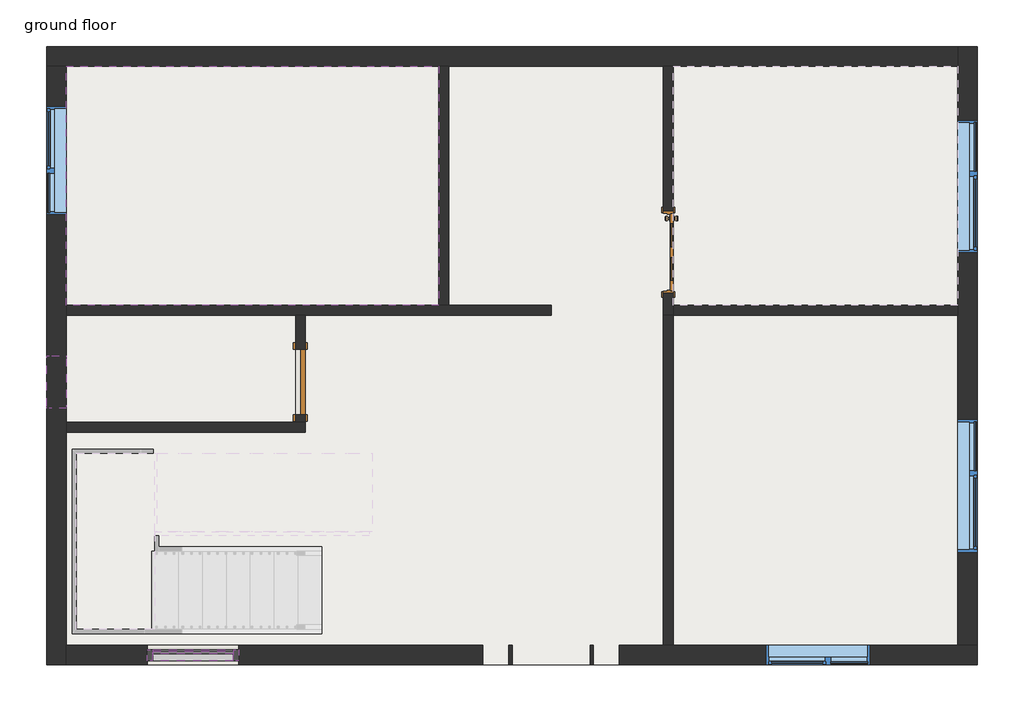
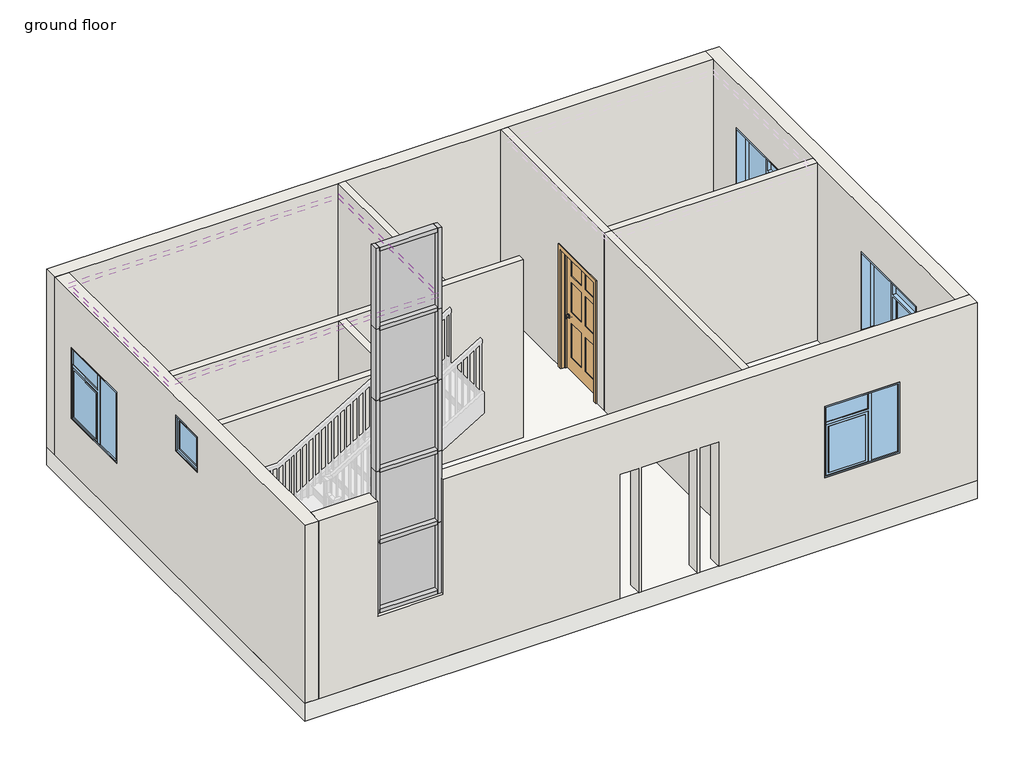
# One storey, part 1 of 3: 16 members, 11 walls, 5 plates, 5 windows, 2 coverings, 2 doors, 1 slab.
"""IFC4 building model written with IfcOpenShell, lengths in millimetres."""

from ifc_helpers import new_model, si_unit, frame, origin, origin_with_axes, place, context, project, spatial, polyline, outline, extrude, faceted_brep, transform, mapped, element, save
from components import door_92bad2d9, door_d8f5dbb5, member_e557a406, member_ca079636, member_75074519, member_331a33ef, system_panel_glazed_b6248f97, system_panel_glazed_e3ab5e3b, system_panel_glazed_f6e6087a, window_80340324, window_ae1cb28a, window_390faff0, window_casement_double_sidelight_windows_4_x_4_2_a48be683

model = new_model("IFC4")

# Units and contexts
model_context = context("Model", 3, world=origin())
ifc_project = project(units=[si_unit("LENGTHUNIT", "METRE", prefix="MILLI")], contexts=[model_context])

# Site, building, storey
site = spatial("IfcSite", under=ifc_project)
building = spatial("IfcBuilding", under=site)
storey = spatial("IfcBuildingStorey", under=building, Name="ground floor", Elevation=304.8)

# Coverings
placement = place(None, origin())
element("IfcCovering", 1, ObjectType="METAL WHITE CEILING", at=placement, inside=storey, context=model_context, shape_type="SweptSolid", body=[
    extrude(outline(polyline([(-15611.0277023, 6236.3679075), (-11248.5777023, 6236.3679075), (-11248.5777023, 3436.0179075), (-15611.0277023, 3436.0179075), (-15611.0277023, 6236.3679075)])), frame((0.0, 0.0, 3175.0), z_axis=(0.0, 0.0, 1.0), x_axis=(1.0, 0.0, 0.0)), (0.0, 0.0, 1.0), 107.95),
])
element("IfcCovering", 2, ObjectType="METAL WHITE CEILING", at=placement, inside=storey, context=model_context, shape_type="SweptSolid", body=[
    extrude(outline(polyline([(-11248.5777023, 6236.3679075), (-11248.5777023, 3436.0179075), (-15611.0277023, 3436.0179075), (-15611.0277023, 6236.3679075), (-11248.5777023, 6236.3679075)]), holes=[polyline([(-11553.3777023, 5931.5679075), (-15306.2277023, 5931.5679075), (-15306.2277023, 3740.8179075), (-11553.3777023, 3740.8179075), (-11553.3777023, 5931.5679075)])]), frame((0.0, 0.0, 3098.8), z_axis=(0.0, 0.0, 1.0), x_axis=(1.0, 0.0, 0.0)), (0.0, 0.0, 1.0), 107.95),
    extrude(outline(polyline([(-14689.9397973, 5626.7679075), (-14689.9397973, 4045.6179075), (-15001.4277023, 4045.6179075), (-15001.4277023, 5626.7679075), (-14689.9397973, 5626.7679075)])), frame((0.0, 0.0, 3098.8), z_axis=(0.0, 0.0, 1.0), x_axis=(1.0, 0.0, 0.0)), (0.0, 0.0, 1.0), 107.95),
    extrude(outline(polyline([(-14080.3397973, 5626.7679075), (-14080.3397973, 4045.6179075), (-14391.8277023, 4045.6179075), (-14391.8277023, 5626.7679075), (-14080.3397973, 5626.7679075)])), frame((0.0, 0.0, 3098.8), z_axis=(0.0, 0.0, 1.0), x_axis=(1.0, 0.0, 0.0)), (0.0, 0.0, 1.0), 107.95),
    extrude(outline(polyline([(-13470.7397973, 5626.7679075), (-13470.7397973, 4045.6179075), (-13782.2277023, 4045.6179075), (-13782.2277023, 5626.7679075), (-13470.7397973, 5626.7679075)])), frame((0.0, 0.0, 3098.8), z_axis=(0.0, 0.0, 1.0), x_axis=(1.0, 0.0, 0.0)), (0.0, 0.0, 1.0), 107.95),
    extrude(outline(polyline([(-12861.1397973, 5626.7679075), (-12861.1397973, 4045.6179075), (-13172.6277023, 4045.6179075), (-13172.6277023, 5626.7679075), (-12861.1397973, 5626.7679075)])), frame((0.0, 0.0, 3098.8), z_axis=(0.0, 0.0, 1.0), x_axis=(1.0, 0.0, 0.0)), (0.0, 0.0, 1.0), 107.95),
    extrude(outline(polyline([(-12251.5397973, 5626.7679075), (-12251.5397973, 4045.6179075), (-12563.0277023, 4045.6179075), (-12563.0277023, 5626.7679075), (-12251.5397973, 5626.7679075)])), frame((0.0, 0.0, 3098.8), z_axis=(0.0, 0.0, 1.0), x_axis=(1.0, 0.0, 0.0)), (0.0, 0.0, 1.0), 107.95),
    extrude(outline(polyline([(-11641.9397973, 5626.7679075), (-11641.9397973, 4045.6179075), (-11953.4277023, 4045.6179075), (-11953.4277023, 5626.7679075), (-11641.9397973, 5626.7679075)])), frame((0.0, 0.0, 3098.8), z_axis=(0.0, 0.0, 1.0), x_axis=(1.0, 0.0, 0.0)), (0.0, 0.0, 1.0), 107.95),
])

# Doors
door_shape = door_92bad2d9(model_context)
element("IfcDoor", 3, ObjectType="Door-Interior-Single-6_Panel-Wood : 36\" x 80\"", at=placement, inside=storey, context=model_context, shape_type="MappedRepresentation", body=[
    mapped(door_shape, transform((-8559.3527023, 4058.3179075, 304.8), x_axis=(0.0, -1.0, 0.0), y_axis=(1.0, 0.0, 0.0), z_axis=(0.0, 0.0, 1.0))),
])
door_2_shape = door_d8f5dbb5(model_context)
element("IfcDoor", 4, ObjectType="Single-Flush : 30\" x 80\"", at=placement, inside=storey, context=model_context, shape_type="MappedRepresentation", body=[
    mapped(door_2_shape, transform((-12867.8277023, 2538.826922, 338.2495969), x_axis=(0.0, -1.0, 0.0), y_axis=(1.0, 0.0, 0.0), z_axis=(0.0, 0.0, 1.0))),
])

# Members
member_shape = member_e557a406(model_context)
element("IfcMember", 5, ObjectType="Rectangular Mullion : 2.5\" x 5\" rectangular", at=placement, inside=storey, context=model_context, shape_type="MappedRepresentation", body=[
    mapped(member_shape, transform((-13655.2277023, -659.7320925, 7647.3395593), x_axis=(0.0, 0.0, 1.0), y_axis=(0.0, -1.0, 0.0), z_axis=(1.0, 0.0, 0.0))),
])
element("IfcMember", 6, ObjectType="Rectangular Mullion : 2.5\" x 5\" rectangular", at=placement, inside=storey, context=model_context, shape_type="MappedRepresentation", body=[
    mapped(member_shape, transform((-14595.0277023, -659.7320925, 1383.1967514), x_axis=(0.0, 0.0, -1.0), y_axis=(0.0, -1.0, 0.0), z_axis=(-1.0, 0.0, 0.0))),
])
member_2_shape = member_ca079636(model_context)
element("IfcMember", 7, ObjectType="Rectangular Mullion : 2.5\" x 5\" rectangular", at=placement, inside=storey, context=model_context, shape_type="MappedRepresentation", body=[
    mapped(member_2_shape, transform((-13655.2277023, -659.7320925, 2602.3967514), x_axis=(0.0, 0.0, 1.0), y_axis=(0.0, -1.0, 0.0), z_axis=(1.0, 0.0, 0.0))),
])
element("IfcMember", 8, ObjectType="Rectangular Mullion : 2.5\" x 5\" rectangular", at=placement, inside=storey, context=model_context, shape_type="MappedRepresentation", body=[
    mapped(member_2_shape, transform((-13655.2277023, -659.7320925, 5040.7967514), x_axis=(0.0, 0.0, 1.0), y_axis=(0.0, -1.0, 0.0), z_axis=(1.0, 0.0, 0.0))),
])
element("IfcMember", 9, ObjectType="Rectangular Mullion : 2.5\" x 5\" rectangular", at=placement, inside=storey, context=model_context, shape_type="MappedRepresentation", body=[
    mapped(member_2_shape, transform((-13655.2277023, -659.7320925, 6259.9967514), x_axis=(0.0, 0.0, 1.0), y_axis=(0.0, -1.0, 0.0), z_axis=(1.0, 0.0, 0.0))),
])
element("IfcMember", 10, ObjectType="Rectangular Mullion : 2.5\" x 5\" rectangular", at=placement, inside=storey, context=model_context, shape_type="MappedRepresentation", body=[
    mapped(member_2_shape, transform((-13655.2277023, -659.7320925, 3821.5967514), x_axis=(0.0, 0.0, 1.0), y_axis=(0.0, -1.0, 0.0), z_axis=(1.0, 0.0, 0.0))),
])
member_3_shape = member_75074519(model_context)
element("IfcMember", 11, ObjectType="Rectangular Mullion : 2.5\" x 5\" rectangular", at=placement, inside=storey, context=model_context, shape_type="MappedRepresentation", body=[
    mapped(member_3_shape, transform((-13591.7277023, -659.7320925, 1383.1967514), x_axis=(1.0, 0.0, 0.0), y_axis=(0.0, -1.0, 0.0), z_axis=(0.0, 0.0, -1.0))),
])
element("IfcMember", 12, ObjectType="Rectangular Mullion : 2.5\" x 5\" rectangular", at=placement, inside=storey, context=model_context, shape_type="MappedRepresentation", body=[
    mapped(member_3_shape, transform((-14658.5277023, -659.7320925, 2602.3967514), x_axis=(-1.0, 0.0, 0.0), y_axis=(0.0, -1.0, 0.0), z_axis=(0.0, 0.0, 1.0))),
])
element("IfcMember", 13, ObjectType="Rectangular Mullion : 2.5\" x 5\" rectangular", at=placement, inside=storey, context=model_context, shape_type="MappedRepresentation", body=[
    mapped(member_3_shape, transform((-14658.5277023, -659.7320925, 3821.5967514), x_axis=(-1.0, 0.0, 0.0), y_axis=(0.0, -1.0, 0.0), z_axis=(0.0, 0.0, 1.0))),
])
element("IfcMember", 14, ObjectType="Rectangular Mullion : 2.5\" x 5\" rectangular", at=placement, inside=storey, context=model_context, shape_type="MappedRepresentation", body=[
    mapped(member_3_shape, transform((-14658.5277023, -659.7320925, 6259.9967514), x_axis=(-1.0, 0.0, 0.0), y_axis=(0.0, -1.0, 0.0), z_axis=(0.0, 0.0, 1.0))),
])
element("IfcMember", 15, ObjectType="Rectangular Mullion : 2.5\" x 5\" rectangular", at=placement, inside=storey, context=model_context, shape_type="MappedRepresentation", body=[
    mapped(member_3_shape, transform((-14658.5277023, -659.7320925, 5040.7967514), x_axis=(-1.0, 0.0, 0.0), y_axis=(0.0, -1.0, 0.0), z_axis=(0.0, 0.0, 1.0))),
])
member_4_shape = member_331a33ef(model_context)
element("IfcMember", 16, ObjectType="Rectangular Mullion : 2.5\" x 5\" rectangular", at=placement, inside=storey, context=model_context, shape_type="MappedRepresentation", body=[
    mapped(member_4_shape, transform((-13591.7277023, -659.7320925, 6259.9967514), x_axis=(1.0, 0.0, 0.0), y_axis=(0.0, -1.0, 0.0), z_axis=(0.0, 0.0, -1.0))),
])
element("IfcMember", 17, ObjectType="Rectangular Mullion : 2.5\" x 5\" rectangular", at=placement, inside=storey, context=model_context, shape_type="MappedRepresentation", body=[
    mapped(member_4_shape, transform((-14658.5277023, -659.7320925, 7647.3395593), x_axis=(-1.0, 0.0, 0.0), y_axis=(0.0, -1.0, 0.0), z_axis=(0.0, 0.0, 1.0))),
])
element("IfcMember", 18, ObjectType="Rectangular Mullion : 2.5\" x 5\" rectangular", at=placement, inside=storey, context=model_context, shape_type="MappedRepresentation", body=[
    mapped(member_3_shape, transform((-13591.7277023, -659.7320925, 3821.5967514), x_axis=(1.0, 0.0, 0.0), y_axis=(0.0, -1.0, 0.0), z_axis=(0.0, 0.0, -1.0))),
])
element("IfcMember", 19, ObjectType="Rectangular Mullion : 2.5\" x 5\" rectangular", at=placement, inside=storey, context=model_context, shape_type="MappedRepresentation", body=[
    mapped(member_3_shape, transform((-13591.7277023, -659.7320925, 2602.3967514), x_axis=(1.0, 0.0, 0.0), y_axis=(0.0, -1.0, 0.0), z_axis=(0.0, 0.0, -1.0))),
])
element("IfcMember", 20, ObjectType="Rectangular Mullion : 2.5\" x 5\" rectangular", at=placement, inside=storey, context=model_context, shape_type="MappedRepresentation", body=[
    mapped(member_3_shape, transform((-13591.7277023, -659.7320925, 5040.7967514), x_axis=(1.0, 0.0, 0.0), y_axis=(0.0, -1.0, 0.0), z_axis=(0.0, 0.0, -1.0))),
])

# Plates
system_panel_glazed_shape = system_panel_glazed_b6248f97(model_context)
element("IfcPlate", 21, ObjectType="System Panel : Glazed", at=placement, inside=storey, context=model_context, shape_type="MappedRepresentation", body=[
    mapped(system_panel_glazed_shape, transform((-14125.1277023, -659.7320925, 1446.6967514), x_axis=(1.0, 0.0, 0.0), y_axis=(0.0, 1.0, 0.0), z_axis=(0.0, 0.0, 1.0))),
])
system_panel_glazed_2_shape = system_panel_glazed_e3ab5e3b(model_context)
element("IfcPlate", 22, ObjectType="System Panel : Glazed", at=placement, inside=storey, context=model_context, shape_type="MappedRepresentation", body=[
    mapped(system_panel_glazed_2_shape, transform((-14125.1277023, -659.7320925, 6291.7467514), x_axis=(1.0, 0.0, 0.0), y_axis=(0.0, 1.0, 0.0), z_axis=(0.0, 0.0, 1.0))),
])
system_panel_glazed_3_shape = system_panel_glazed_f6e6087a(model_context)
element("IfcPlate", 23, ObjectType="System Panel : Glazed", at=placement, inside=storey, context=model_context, shape_type="MappedRepresentation", body=[
    mapped(system_panel_glazed_3_shape, transform((-14125.1277023, -659.7320925, 3853.3467514), x_axis=(1.0, 0.0, 0.0), y_axis=(0.0, 1.0, 0.0), z_axis=(0.0, 0.0, 1.0))),
])
element("IfcPlate", 24, ObjectType="System Panel : Glazed", at=placement, inside=storey, context=model_context, shape_type="MappedRepresentation", body=[
    mapped(system_panel_glazed_3_shape, transform((-14125.1277023, -659.7320925, 2634.1467514), x_axis=(1.0, 0.0, 0.0), y_axis=(0.0, 1.0, 0.0), z_axis=(0.0, 0.0, 1.0))),
])
element("IfcPlate", 25, ObjectType="System Panel : Glazed", at=placement, inside=storey, context=model_context, shape_type="MappedRepresentation", body=[
    mapped(system_panel_glazed_3_shape, transform((-14125.1277023, -659.7320925, 5072.5467514), x_axis=(1.0, 0.0, 0.0), y_axis=(0.0, 1.0, 0.0), z_axis=(0.0, 0.0, 1.0))),
])

# Slab
element("IfcSlab", 26, ObjectType="FLOORING 1'", at=placement, inside=storey, context=model_context, shape_type="SweptSolid", body=[
    extrude(outline(polyline([(-4943.0277023, 6464.9679075), (-4943.0277023, -774.0320925), (-15839.6277023, -774.0320925), (-15839.6277023, 6464.9679075), (-4943.0277023, 6464.9679075)])), origin_with_axes(), (0.0, 0.0, 1.0), 304.8),
])

# Walls
element("IfcWall", 27, ObjectType="OUTER Wall 9\"", at=placement, inside=storey, context=model_context, shape_type="Brep", body=[
    faceted_brep([(-15839.6277023, 6236.3679075, 304.8), (-15611.0277023, 6236.3679075, 304.8), (-11248.5777023, 6236.3679075, 304.8), (-11134.2777023, 6236.3679075, 304.8), (-8619.6777023, 6236.3679075, 304.8), (-8505.3777023, 6236.3679075, 304.8), (-5171.6277023, 6236.3679075, 304.8), (-5171.6277023, 6236.3679075, 3352.8), (-8505.3777023, 6236.3679075, 3352.8), (-8619.6777023, 6236.3679075, 3352.8), (-11134.2777023, 6236.3679075, 3352.8), (-11248.5777023, 6236.3679075, 3352.8), (-15611.0277023, 6236.3679075, 3352.8), (-15839.6277023, 6236.3679075, 3352.8), (-15839.6277023, 6464.9679075, 304.8), (-15839.6277023, 6464.9679075, 3352.8), (-5171.6277023, 6464.9679075, 3352.8), (-5171.6277023, 6464.9679075, 304.8)], [[[0, 1, 2, 3, 4, 5, 6, 7, 8, 9, 10, 11, 12, 13]], [[14, 15, 16, 17]], [[6, 5, 4, 3, 2, 1, 0, 14, 17]], [[13, 12, 11, 10, 9, 8, 7, 16, 15]], [[0, 13, 15, 14]], [[7, 6, 17, 16]]]),
])
element("IfcWall", 28, ObjectType="OUTER Wall 9\"", at=placement, inside=storey, context=model_context, shape_type="Brep", body=[
    faceted_brep([(-15611.0277023, -774.0320925, 304.8), (-15611.0277023, -545.4320925, 304.8), (-15611.0277023, 1950.1179075, 304.8), (-15611.0277023, 2064.4179075, 304.8), (-15611.0277023, 3321.7179075, 304.8), (-15611.0277023, 3436.0179075, 304.8), (-15611.0277023, 6236.3679075, 304.8), (-15611.0277023, 6236.3679075, 3352.8), (-15611.0277023, 3436.0179075, 3352.8), (-15611.0277023, 3321.7179075, 3352.8), (-15611.0277023, 2064.4179075, 3352.8), (-15611.0277023, 1950.1179075, 3352.8), (-15611.0277023, -545.4320925, 3352.8), (-15611.0277023, -774.0320925, 3352.8), (-15611.0277023, 2842.7064293, 3048.0), (-15611.0277023, 2842.7064293, 2438.4), (-15611.0277023, 2233.1064293, 2438.4), (-15611.0277023, 2233.1064293, 3048.0), (-15611.0277023, 5766.4679075, 2438.4), (-15611.0277023, 5766.4679075, 1219.2), (-15611.0277023, 4496.4679075, 1219.2), (-15611.0277023, 4496.4679075, 2438.4), (-15839.6277023, 6236.3679075, 304.8), (-15839.6277023, -774.0320925, 304.8), (-15839.6277023, -774.0320925, 3352.8), (-15839.6277023, 6236.3679075, 3352.8), (-15839.6277023, 2842.7064293, 2438.4), (-15839.6277023, 2842.7064293, 3048.0), (-15839.6277023, 2233.1064293, 3048.0), (-15839.6277023, 2233.1064293, 2438.4), (-15839.6277023, 5766.4679075, 1219.2), (-15839.6277023, 5766.4679075, 2438.4), (-15839.6277023, 4496.4679075, 2438.4), (-15839.6277023, 4496.4679075, 1219.2)], [[[0, 1, 2, 3, 4, 5, 6, 7, 8, 9, 10, 11, 12, 13], [14, 15, 16, 17], [18, 19, 20, 21]], [[22, 23, 24, 25], [26, 27, 28, 29], [30, 31, 32, 33]], [[6, 5, 4, 3, 2, 1, 0, 23, 22]], [[13, 12, 11, 10, 9, 8, 7, 25, 24]], [[0, 13, 24, 23]], [[7, 6, 22, 25]], [[14, 27, 26, 15]], [[15, 26, 29, 16]], [[16, 29, 28, 17]], [[27, 14, 17, 28]], [[19, 18, 31, 30]], [[20, 19, 30, 33]], [[21, 20, 33, 32]], [[18, 21, 32, 31]]]),
])
element("IfcWall", 29, ObjectType="OUTER Wall 9\"", at=placement, inside=storey, context=model_context, shape_type="Brep", body=[
    faceted_brep([(-4943.0277023, -545.4320925, 3352.8), (-4943.0277023, -545.4320925, 304.8), (-5171.6277023, -545.4320925, 304.8), (-8505.3777023, -545.4320925, 304.8), (-8619.6777023, -545.4320925, 304.8), (-9134.0277023, -545.4320925, 304.8), (-9134.0277023, -545.4320925, 2438.4), (-9438.8277023, -545.4320925, 2438.4), (-9438.8277023, -545.4320925, 304.8), (-9476.9277023, -545.4320925, 304.8), (-9476.9277023, -545.4320925, 2438.4), (-10391.3277023, -545.4320925, 2438.4), (-10391.3277023, -545.4320925, 304.8), (-10429.4277023, -545.4320925, 304.8), (-10429.4277023, -545.4320925, 2438.4), (-10734.2277023, -545.4320925, 2438.4), (-10734.2277023, -545.4320925, 304.8), (-15611.0277023, -545.4320925, 304.8), (-15611.0277023, -545.4320925, 3352.8), (-14658.5277023, -545.4320925, 3352.8), (-14658.5277023, -545.4320925, 1383.1967514), (-13591.7277023, -545.4320925, 1383.1967514), (-13591.7277023, -545.4320925, 3352.8), (-8619.6777023, -545.4320925, 3352.8), (-8505.3777023, -545.4320925, 3352.8), (-5171.6277023, -545.4320925, 3352.8), (-7419.5277023, -545.4320925, 2438.4), (-7419.5277023, -545.4320925, 1219.2), (-6200.3277023, -545.4320925, 1219.2), (-6200.3277023, -545.4320925, 2438.4), (-4943.0277023, -774.0320925, 304.8), (-4943.0277023, -774.0320925, 3352.8), (-13591.7277023, -774.0320925, 3352.8), (-13591.7277023, -774.0320925, 1383.1967514), (-14658.5277023, -774.0320925, 1383.1967514), (-14658.5277023, -774.0320925, 3352.8), (-15611.0277023, -774.0320925, 3352.8), (-15611.0277023, -774.0320925, 304.8), (-10734.2277023, -774.0320925, 304.8), (-10734.2277023, -774.0320925, 2438.4), (-10429.4277023, -774.0320925, 2438.4), (-10429.4277023, -774.0320925, 304.8), (-10391.3277023, -774.0320925, 304.8), (-10391.3277023, -774.0320925, 2438.4), (-9476.9277023, -774.0320925, 2438.4), (-9476.9277023, -774.0320925, 304.8), (-9438.8277023, -774.0320925, 304.8), (-9438.8277023, -774.0320925, 2438.4), (-9134.0277023, -774.0320925, 2438.4), (-9134.0277023, -774.0320925, 304.8), (-7419.5277023, -774.0320925, 2438.4), (-6200.3277023, -774.0320925, 2438.4), (-6200.3277023, -774.0320925, 1219.2), (-7419.5277023, -774.0320925, 1219.2)], [[[0, 1, 2, 3, 4, 5, 6, 7, 8, 9, 10, 11, 12, 13, 14, 15, 16, 17, 18, 19, 20, 21, 22, 23, 24, 25], [26, 27, 28, 29]], [[30, 31, 32, 33, 34, 35, 36, 37, 38, 39, 40, 41, 42, 43, 44, 45, 46, 47, 48, 49], [50, 51, 52, 53]], [[1, 30, 49, 5, 4, 3, 2]], [[37, 17, 16, 38]], [[12, 42, 41, 13]], [[45, 9, 8, 46]], [[31, 0, 25, 24, 23, 22, 32]], [[18, 36, 35, 19]], [[1, 0, 31, 30]], [[18, 17, 37, 36]], [[12, 11, 43, 42]], [[11, 10, 44, 43]], [[10, 9, 45, 44]], [[39, 38, 16, 15]], [[40, 39, 15, 14]], [[41, 40, 14, 13]], [[6, 5, 49, 48]], [[7, 6, 48, 47]], [[8, 7, 47, 46]], [[27, 26, 50, 53]], [[28, 27, 53, 52]], [[29, 28, 52, 51]], [[26, 29, 51, 50]], [[34, 20, 19, 35]], [[21, 33, 32, 22]], [[20, 34, 33, 21]]]),
])
element("IfcWall", 30, ObjectType="OUTER Wall 9\"", at=placement, inside=storey, context=model_context, shape_type="Brep", body=[
    faceted_brep([(-5171.6277023, 6464.9679075, 304.8), (-5171.6277023, 6236.3679075, 304.8), (-5171.6277023, 3436.0179075, 304.8), (-5171.6277023, 3321.7179075, 304.8), (-5171.6277023, -545.4320925, 304.8), (-5171.6277023, -545.4320925, 3352.8), (-5171.6277023, 3321.7179075, 3352.8), (-5171.6277023, 3436.0179075, 3352.8), (-5171.6277023, 6236.3679075, 3352.8), (-5171.6277023, 6464.9679075, 3352.8), (-5171.6277023, 546.7679075, 2565.4), (-5171.6277023, 546.7679075, 1219.2), (-5171.6277023, 2096.1679075, 1219.2), (-5171.6277023, 2096.1679075, 2565.4), (-5171.6277023, 4051.9679075, 2565.4), (-5171.6277023, 4051.9679075, 1219.2), (-5171.6277023, 5601.3679075, 1219.2), (-5171.6277023, 5601.3679075, 2565.4), (-4943.0277023, 6464.9679075, 304.8), (-4943.0277023, 6464.9679075, 3352.8), (-4943.0277023, -545.4320925, 3352.8), (-4943.0277023, -545.4320925, 304.8), (-4943.0277023, 546.7679075, 2565.4), (-4943.0277023, 2096.1679075, 2565.4), (-4943.0277023, 2096.1679075, 1219.2), (-4943.0277023, 546.7679075, 1219.2), (-4943.0277023, 4051.9679075, 2565.4), (-4943.0277023, 5601.3679075, 2565.4), (-4943.0277023, 5601.3679075, 1219.2), (-4943.0277023, 4051.9679075, 1219.2)], [[[0, 1, 2, 3, 4, 5, 6, 7, 8, 9], [10, 11, 12, 13], [14, 15, 16, 17]], [[18, 19, 20, 21], [22, 23, 24, 25], [26, 27, 28, 29]], [[4, 3, 2, 1, 0, 18, 21]], [[9, 8, 7, 6, 5, 20, 19]], [[0, 9, 19, 18]], [[5, 4, 21, 20]], [[11, 10, 22, 25]], [[12, 11, 25, 24]], [[13, 12, 24, 23]], [[10, 13, 23, 22]], [[15, 14, 26, 29]], [[16, 15, 29, 28]], [[17, 16, 28, 27]], [[14, 17, 27, 26]]]),
])
element("IfcWall", 31, ObjectType="inner wall 4.5\"", at=placement, inside=storey, context=model_context, shape_type="SweptSolid", body=[
    extrude(outline(polyline([(-8505.3777023, 3321.7179075), (-8505.3777023, -545.4320925), (-8619.6777023, -545.4320925), (-8619.6777023, 3321.7179075), (-8505.3777023, 3321.7179075)])), frame((0.0, 0.0, 304.8), z_axis=(0.0, 0.0, 1.0), x_axis=(1.0, 0.0, 0.0)), (0.0, 0.0, 1.0), 3048.0),
])
element("IfcWall", 32, ObjectType="inner wall 4.5\"", at=placement, inside=storey, context=model_context, shape_type="Brep", body=[
    faceted_brep([(-9934.1277023, 3436.0179075, 304.8), (-11134.2777023, 3436.0179075, 304.8), (-11248.5777023, 3436.0179075, 304.8), (-15611.0277023, 3436.0179075, 304.8), (-15611.0277023, 3436.0179075, 3352.8), (-11248.5777023, 3436.0179075, 3352.8), (-11134.2777023, 3436.0179075, 3352.8), (-9934.1277023, 3436.0179075, 3352.8), (-9934.1277023, 3321.7179075, 304.8), (-9934.1277023, 3321.7179075, 3352.8), (-12810.6777023, 3321.7179075, 3352.8), (-12924.9777023, 3321.7179075, 3352.8), (-15611.0277023, 3321.7179075, 3352.8), (-15611.0277023, 3321.7179075, 304.8), (-12924.9777023, 3321.7179075, 304.8), (-12810.6777023, 3321.7179075, 304.8)], [[[0, 1, 2, 3, 4, 5, 6, 7]], [[8, 9, 10, 11, 12, 13, 14, 15]], [[3, 2, 1, 0, 8, 15, 14, 13]], [[7, 6, 5, 4, 12, 11, 10, 9]], [[0, 7, 9, 8]], [[4, 3, 13, 12]]]),
])
element("IfcWall", 33, ObjectType="inner wall 4.5\"", at=placement, inside=storey, context=model_context, shape_type="Brep", body=[
    faceted_brep([(-8619.6777023, 3321.7179075, 3352.8), (-8619.6777023, 6236.3679075, 3352.8), (-8619.6777023, 6236.3679075, 304.8), (-8619.6777023, 4540.9179075, 304.8), (-8619.6777023, 4540.9179075, 2362.2), (-8619.6777023, 3575.7179075, 2362.2), (-8619.6777023, 3575.7179075, 304.8), (-8619.6777023, 3321.7179075, 304.8), (-8505.3777023, 6236.3679075, 3352.8), (-8505.3777023, 3436.0179075, 3352.8), (-8505.3777023, 3321.7179075, 3352.8), (-8505.3777023, 3321.7179075, 304.8), (-8505.3777023, 3436.0179075, 304.8), (-8505.3777023, 3575.7179075, 304.8), (-8505.3777023, 3575.7179075, 2362.2), (-8505.3777023, 4540.9179075, 2362.2), (-8505.3777023, 4540.9179075, 304.8), (-8505.3777023, 6236.3679075, 304.8)], [[[0, 1, 2, 3, 4, 5, 6, 7]], [[8, 9, 10, 11, 12, 13, 14, 15, 16, 17]], [[2, 17, 16, 3]], [[11, 7, 6, 13, 12]], [[1, 0, 10, 9, 8]], [[2, 1, 8, 17]], [[0, 7, 11, 10]], [[5, 14, 13, 6]], [[14, 5, 4, 15]], [[15, 4, 3, 16]]]),
])
element("IfcWall", 34, ObjectType="inner wall 4.5\"", at=placement, inside=storey, context=model_context, shape_type="Brep", body=[
    faceted_brep([(-15611.0277023, 1950.1179075, 304.8), (-12810.6777023, 1950.1179075, 304.8), (-12810.6777023, 1950.1179075, 3352.8), (-15611.0277023, 1950.1179075, 3352.8), (-15611.0277023, 2064.4179075, 304.8), (-15611.0277023, 2064.4179075, 3352.8), (-12924.9777023, 2064.4179075, 3352.8), (-12810.6777023, 2064.4179075, 3352.8), (-12810.6777023, 2064.4179075, 304.8), (-12924.9777023, 2064.4179075, 304.8)], [[[0, 1, 2, 3]], [[4, 5, 6, 7, 8, 9]], [[1, 0, 4, 9, 8]], [[3, 2, 7, 6, 5]], [[0, 3, 5, 4]], [[2, 1, 8, 7]]]),
])
element("IfcWall", 35, ObjectType="inner wall 4.5\"", at=placement, inside=storey, context=model_context, shape_type="SweptSolid", body=[
    extrude(outline(polyline([(3321.7179075, 304.8), (2064.4179075, 304.8), (2064.4179075, 3352.8), (3321.7179075, 3352.8), (3321.7179075, 304.8)]), holes=[polyline([(2157.826922, 338.2495969), (2919.826922, 338.2495969), (2919.826922, 2370.2495969), (2157.826922, 2370.2495969), (2157.826922, 338.2495969)])]), frame((-12924.9777023, 0.0, 0.0), z_axis=(1.0, 0.0, 0.0), x_axis=(0.0, 1.0, 0.0)), (0.0, 0.0, 1.0), 114.3),
])
element("IfcWall", 36, ObjectType="inner wall 4.5\"", at=placement, inside=storey, context=model_context, shape_type="SweptSolid", body=[
    extrude(outline(polyline([(-8505.3777023, 3436.0179075), (-5171.6277023, 3436.0179075), (-5171.6277023, 3321.7179075), (-8505.3777023, 3321.7179075), (-8505.3777023, 3436.0179075)])), frame((0.0, 0.0, 304.8), z_axis=(0.0, 0.0, 1.0), x_axis=(1.0, 0.0, 0.0)), (0.0, 0.0, 1.0), 3048.0),
])
element("IfcWall", 37, ObjectType="inner wall 4.5\"", at=placement, inside=storey, context=model_context, shape_type="SweptSolid", body=[
    extrude(outline(polyline([(-11248.5777023, 3436.0179075), (-11248.5777023, 6236.3679075), (-11134.2777023, 6236.3679075), (-11134.2777023, 3436.0179075), (-11248.5777023, 3436.0179075)])), frame((0.0, 0.0, 304.8), z_axis=(0.0, 0.0, 1.0), x_axis=(1.0, 0.0, 0.0)), (0.0, 0.0, 1.0), 3048.0),
])

# Windows
window_shape = window_80340324(model_context)
element("IfcWindow", 38, ObjectType="Fixed : 24\" x 24\"", at=placement, inside=storey, context=model_context, shape_type="MappedRepresentation", body=[
    mapped(window_shape, transform((-15725.3277023, 2576.0064293, 1524.0), x_axis=(0.0, 1.0, 0.0), y_axis=(-1.0, 0.0, 0.0), z_axis=(0.0, 0.0, 1.0))),
])
window_2_shape = window_ae1cb28a(model_context)
element("IfcWindow", 39, ObjectType="Window-Casement-Double-Sidelight : 50\" x 48\"", at=placement, inside=storey, context=model_context, shape_type="MappedRepresentation", body=[
    mapped(window_2_shape, transform((-15725.3277023, 5131.4679075, 304.8), x_axis=(0.0, 1.0, 0.0), y_axis=(-1.0, 0.0, 0.0), z_axis=(0.0, 0.0, 1.0))),
])
window_3_shape = window_390faff0(model_context)
element("IfcWindow", 40, ObjectType="Window-Casement-Double-Sidelight : 61\" x 53\"", at=placement, inside=storey, context=model_context, shape_type="MappedRepresentation", body=[
    mapped(window_3_shape, transform((-5057.3277023, 1321.4679075, 304.8), x_axis=(0.0, -1.0, 0.0), y_axis=(1.0, 0.0, 0.0), z_axis=(0.0, 0.0, 1.0))),
])
element("IfcWindow", 41, ObjectType="Window-Casement-Double-Sidelight : 61\" x 53\"", at=placement, inside=storey, context=model_context, shape_type="MappedRepresentation", body=[
    mapped(window_3_shape, transform((-5057.3277023, 4826.6679075, 304.8), x_axis=(0.0, -1.0, 0.0), y_axis=(1.0, 0.0, 0.0), z_axis=(0.0, 0.0, 1.0))),
])
window_casement_double_sidelight_windows_4_x_4_2_shape = window_casement_double_sidelight_windows_4_x_4_2_a48be683(model_context)
element("IfcWindow", 42, ObjectType="Window-Casement-Double-Sidelight : WINDOWS 4' X 4' 2", at=placement, inside=storey, context=model_context, shape_type="MappedRepresentation", body=[
    mapped(window_casement_double_sidelight_windows_4_x_4_2_shape, transform((-6809.9277023, -659.7320925, 304.8), x_axis=(-1.0, 0.0, 0.0), y_axis=(0.0, -1.0, 0.0), z_axis=(0.0, 0.0, 1.0))),
])

save(model, "model.ifc")

# Revit data of these elements
# Type "METAL WHITE CEILING"
#   Assembly Code = "C3030220"
#   built-in parameter 1002203 = 1 (stored number, unit not read)
#   built-in parameter 1002202 = 1 (stored number, unit not read)
#   Layers, outside or top first: 0' - 3 5/8" "Metal Stud Layer" (function 1); 0' - 0 5/8" "Laminate, Ivory, Matte" (function 5)
# Type "Door-Interior-Single-6_Panel-Wood : 36\" x 80\""
#   Type Mark = "10"
#   Assembly Code = "C1020300"
#   Analytic Construction = "Wooden"
#   Top Rail = 0' - 4 11/16"
#   Top Panel = 0' - 11"
#   Thickness = 0' - 1 3/8"
#   Thermal Resistance (R) = 2.5876 (h·ft²·°F)/BTU
#   Swing Angle [instance default] = 90.00°
#   Stiles = 0' - 4 3/4"
#   Rough Width = 3' - 2"
#   Rough Height = 6' - 9"
#   Mullion = 0' - 4 1/2"
#   Lock Rail = 0' - 7 1/2"
#   Intermediate Rail = 0' - 4 1/2"
#   Height = 6' - 8"
#   Width = 3' - 0"
#   Heat Transfer Coefficient (U) = 0.3865 BTU/(h·ft²·°F)
#   Bottom Rail = 0' - 9 1/8"
#   Trim Material = Cherry
#   Panel Material = Cherry
#   Frame Material = Cherry
#   Door Handle Material = Aluminum
#   Visual Light Transmittance = 0
#   Solar Heat Gain Coefficient = 0
#   Wall Closure = (empty or 0)
#   Function = (empty or 0)
# Type "Single-Flush : 30\" x 80\""
#   Type Mark = "5"
#   Construction Type Id = "MDOOR"
#   Assembly Code = "C1020"
#   Analytic Construction = "Metal"
#   Thickness = 0' - 2"
#   Heat Transfer Coefficient (U) = 0.651978 BTU/(h·ft²·°F)
#   Height = 6' - 8"
#   Trim Projection Ext = 0' - 1"
#   Trim Projection Int = 0' - 1"
#   Trim Width = 0' - 3"
#   Width = 2' - 6"
#   Define Thermal Properties by = 1
#   Define Thermal Properties by = 1
#   Door Material = Door - Panel
#   Frame Material = Door - Frame
#   Visual Light Transmittance = 0
#   Solar Heat Gain Coefficient = 0
#   Function = (empty or 0)
#   Wall Closure = (empty or 0)
# Type "Rectangular Mullion : 2.5\" x 5\" rectangular"
#   built-in parameter 1007304 = 0.416667 (stored number, unit not read)
#   built-in parameter 1007301 = 0.104167 (stored number, unit not read)
#   built-in parameter 1007300 = 0.104167 (stored number, unit not read)
# Type "System Panel : Glazed"
#   Construction Type Id = "GSP4R"
#   Analytic Construction = "1/8 in Pilkington single glazing"
#   Visual Light Transmittance = 0.9
#   Solar Heat Gain Coefficient = 0.86
#   Heat Transfer Coefficient (U) = 1.18115 BTU/(h·ft²·°F)
#   Define Thermal Properties by = 1
# Type "FLOORING 1'"
#   Assembly Code = "B1010"
#   Function = 0
#   Layers, outside or top first: 1' - 0" "FLOORING 1'" (function 1)
# Type "OUTER Wall 9\""
#   Assembly Code = "B2010"
#   Layers, outside or top first: 0' - 9" "outer wall" (function 1)
# Type "inner wall 4.5\""
#   Assembly Code = "B2010"
#   Layers, outside or top first: 0' - 4 1/2" "outer wall" (function 1)
# Type "Fixed : 24\" x 24\""
#   Type Mark = "3"
#   Construction Type Id = "GSP4R"
#   Assembly Code = "B2020100"
#   Analytic Construction = "1/8 in Pilkington single glazing"
#   Visual Light Transmittance = 0.9
#   Solar Heat Gain Coefficient = 0.78
#   Heat Transfer Coefficient (U) = 0.6496 BTU/(h·ft²·°F)
#   Height = 2' - 0"
#   Default Sill Height = 3' - 0"
#   Width = 2' - 0"
#   Window Inset = 0' - 0 3/4"
#   Define Thermal Properties by = 1
#   Define Thermal Properties by = 1
#   Glass Pane Material = Glass
#   Sash Material = Sash
#   Wall Closure = (empty or 0)
# Type "Window-Casement-Double-Sidelight : 50\" x 48\""
#   Type Mark = "22"
#   Fire Rating = "0.5h"
#   Assembly Code = "B2020100"
#   Analytic Construction = "Double glazing - domestic"
#   Window Inset [instance default] = 0' - 0 5/8"
#   Wall Thickness [instance default] = 0' - 6"
#   Visual Light Transmittance = 0.81
#   Transom Height Ratio = 0.25
#   Transom Height = 1' - 0"
#   Thermal Resistance (R) = 1.8146 (h·ft²·°F)/BTU
#   Solar Heat Gain Coefficient = 0.76
#   Side Width = 1' - 8"
#   Rough Width = 4' - 2 1/2"
#   Rough Height = 4' - 0 1/2"
#   Opening Window Width = 2' - 6"
#   Opening Window Height = 3' - 0"
#   Heat Transfer Coefficient (U) = 0.5511 BTU/(h·ft²·°F)
#   Height = 4' - 0"
#   Frame Gap 3 [instance default] = 0' - 1 83/128"
#   Frame Gap 2 [instance default] = 0' - 0 5/8"
#   Frame Gap 1 = 0' - 1 51/128"
#   Default Sill Height = 3' - 0"
#   Width = 4' - 2"
#   Frame Material = Metal - Aluminum
#   Glass Panel Material = Glass
#   Wall Closure = (empty or 0)
# Type "Window-Casement-Double-Sidelight : 61\" x 53\""
#   Type Mark = "21"
#   Fire Rating = "0.5h"
#   Assembly Code = "B2020100"
#   Analytic Construction = "Double glazing - domestic"
#   Window Inset [instance default] = 0' - 0 5/8"
#   Wall Thickness [instance default] = 0' - 6"
#   Visual Light Transmittance = 0.81
#   Transom Height Ratio = 0.3
#   Transom Height = 1' - 3.9"
#   Thermal Resistance (R) = 1.8146 (h·ft²·°F)/BTU
#   Solar Heat Gain Coefficient = 0.76
#   Side Width = 2' - 0.4"
#   Rough Width = 5' - 1 1/2"
#   Rough Height = 4' - 5 1/2"
#   Opening Window Width = 3' - 0.6"
#   Opening Window Height = 3' - 1.1"
#   Heat Transfer Coefficient (U) = 0.5511 BTU/(h·ft²·°F)
#   Height = 4' - 5"
#   Frame Gap 3 [instance default] = 0' - 1 83/128"
#   Frame Gap 2 [instance default] = 0' - 0 5/8"
#   Frame Gap 1 = 0' - 1 51/128"
#   Default Sill Height = 3' - 0"
#   Width = 5' - 1"
#   Frame Material = Metal - Aluminum
#   Glass Panel Material = Glass
#   Wall Closure = (empty or 0)
# Type "Window-Casement-Double-Sidelight : WINDOWS 4' X 4' 2"
#   Type Mark = "25"
#   Fire Rating = "0.5h"
#   Assembly Code = "B2020100"
#   Analytic Construction = "Double glazing - domestic"
#   Window Inset [instance default] = 0' - 0 5/8"
#   Wall Thickness [instance default] = 0' - 6"
#   Visual Light Transmittance = 0.81
#   Transom Height Ratio = 0.25
#   Transom Height = 1' - 0"
#   Thermal Resistance (R) = 1.8146 (h·ft²·°F)/BTU
#   Solar Heat Gain Coefficient = 0.76
#   Side Width = 1' - 7.2"
#   Rough Width = 4' - 0 1/2"
#   Rough Height = 4' - 0 1/2"
#   Opening Window Width = 2' - 4.8"
#   Opening Window Height = 3' - 0"
#   Heat Transfer Coefficient (U) = 0.5511 BTU/(h·ft²·°F)
#   Height = 4' - 0"
#   Frame Gap 3 [instance default] = 0' - 1 83/128"
#   Frame Gap 2 [instance default] = 0' - 0 5/8"
#   Frame Gap 1 = 0' - 1 51/128"
#   Default Sill Height = 3' - 0"
#   Width = 4' - 0"
#   Frame Material = BLACK MATERIAL
#   Glass Panel Material = Glass
#   Wall Closure = (empty or 0)
# Element 1 (IfcCovering, "METAL WHITE CEILING")
#   Height Offset From Level = 9' - 5"
#   Phase Created = New Construction
#   Materials on its faces: "Laminate, Ivory, Matte", "Metal Stud Layer"
# Element 2 (IfcCovering, "METAL WHITE CEILING")
#   Height Offset From Level = 9' - 2"
#   Phase Created = New Construction
#   Materials on its faces: "Laminate, Ivory, Matte", "Metal Stud Layer"
# Element 3 (IfcDoor, "Door-Interior-Single-6_Panel-Wood : 36\" x 80\"")
#   Swing Angle = 90.00°
#   Phase Created = New Construction
#   Materials on its faces: "Cherry", "Aluminum"
# Element 4 (IfcDoor, "Single-Flush : 30\" x 80\"")
#   Phase Created = New Construction
#   Materials on its faces: "Door - Frame", "Door - Panel"
# Elements 5, 6, 7, 8, 9, 10, 11, 12, 13, 14, 15, 16, 17, 18, 19, 20 (IfcMember, "Rectangular Mullion : 2.5\" x 5\" rectangular")
#   Phase Created = New Construction
#   Materials on its faces: "Aluminum"
# Elements 21, 22, 23, 24, 25 (IfcPlate, "System Panel : Glazed")
#   Phase Created = New Construction
#   Materials on its faces: "Glass"
# Element 26 (IfcSlab, "FLOORING 1'")
#   Height Offset From Level = 0' - 0"
#   Phase Created = New Construction
#   Materials on its faces: "FLOORING 1'"
# Elements 27, 28, 29, 30 (IfcWall, "OUTER Wall 9\"")
#   Top Offset = 0' - 0"
#   Base Offset = 0' - 0"
#   wall height = 10' - 0"
#   Phase Created = New Construction
#   Base Constraint = ground floor
#   Top Constraint = Level 2
#   Materials on its faces: "outer wall"
# Elements 31, 32, 33, 34, 35, 36, 37 (IfcWall, "inner wall 4.5\"")
#   Top Offset = 0' - 0"
#   Base Offset = 0' - 0"
#   wall height = 10' - 0"
#   Phase Created = New Construction
#   Base Constraint = ground floor
#   Top Constraint = Level 2
#   Materials on its faces: "outer wall"
# Element 38 (IfcWindow, "Fixed : 24\" x 24\"")
#   Mark = "1"
#   Phase Created = New Construction
#   Materials on its faces: "Sash", "Glass"
# Element 39 (IfcWindow, "Window-Casement-Double-Sidelight : 50\" x 48\"")
#   Mark = "5"
#   Window Inset = 0' - 0 5/8"
#   Frame Gap 3 = 0' - 1 83/128"
#   Frame Gap 2 = 0' - 0 5/8"
#   Phase Created = New Construction
#   Materials on its faces: "Metal - Aluminum", "Glass"
# Element 40 (IfcWindow, "Window-Casement-Double-Sidelight : 61\" x 53\"")
#   Mark = "3"
#   Window Inset = 0' - 0 5/8"
#   Frame Gap 3 = 0' - 1 83/128"
#   Frame Gap 2 = 0' - 0 5/8"
#   Phase Created = New Construction
#   Materials on its faces: "Metal - Aluminum", "Glass"
# Element 41 (IfcWindow, "Window-Casement-Double-Sidelight : 61\" x 53\"")
#   Mark = "4"
#   Window Inset = 0' - 0 5/8"
#   Frame Gap 3 = 0' - 1 83/128"
#   Frame Gap 2 = 0' - 0 5/8"
#   Phase Created = New Construction
#   Materials on its faces: "Metal - Aluminum", "Glass"
# Element 42 (IfcWindow, "Window-Casement-Double-Sidelight : WINDOWS 4' X 4' 2")
#   Mark = "6"
#   Window Inset = 0' - 0 5/8"
#   Frame Gap 3 = 0' - 1 83/128"
#   Frame Gap 2 = 0' - 0 5/8"
#   Phase Created = New Construction
#   Materials on its faces: "BLACK MATERIAL", "Glass"
# Materials
#   "Metal Stud Layer": class "Metal", colour RGB 199 199 199, transparency 0, Description = "Light gauge steel framing, thermal air layer", Cost = 0
#   "Laminate, Ivory, Matte": class "Plastic", colour RGB 247 247 239, transparency 0, Description = "Plastic Laminate - Ivory, Matte", Cost = 0
#   "Cherry": class "Wood", colour RGB 226 177 128, transparency 0, Description = "Prunus Serotina", Cost = 0
#   "Aluminum": class "Metal", colour RGB 247 247 247, transparency 0, Description = "Aluminum 6061", Cost = 0
#   "Door - Panel": class "Wood", colour RGB 210 159 95, transparency 0, Cost = 0
#   "Door - Frame": colour RGB 118 70 51, transparency 0, Cost = 0
#   "FLOORING 1'": class "Generic", colour RGB 120 120 120, transparency 0, Cost = 0
#   "outer wall": class "Generic", colour RGB 120 120 120, transparency 0, Cost = 0
#   "Glass": class "Glass", colour RGB 0 128 192, transparency 0.75, Description = "Soda Lime Glass", Cost = 0
#   "Sash": class "Wood", colour RGB 224 178 126, transparency 0, Cost = 0
#   "Metal - Aluminum": class "Metal", colour RGB 247 247 247, transparency 0
#   "BLACK MATERIAL": class "Generic", colour RGB 120 120 120, transparency 0, Cost = 0
# Room at (-14296.578, 2693.068) mm, phase "New Construction", upper level "ground floor", upper offset 10' - 0", lower offset 0' - 0"
#   Number = "1"
#   Name = "TOILET"
# Room at (-6809.928, 1626.268) mm, phase "New Construction", upper level "ground floor", upper offset 10' - 0", lower offset 0' - 0"
#   Number = "2"
#   Name = "KITCHEN"
# Room at (-6809.928, 4902.868) mm, phase "New Construction", upper level "ground floor", upper offset 10' - 0", lower offset 0' - 0"
#   Number = "3"
#   Name = "GUEST ROOM"
# Room at (-12143.928, 4902.868) mm, phase "New Construction", upper level "ground floor", upper offset 10' - 0", lower offset 0' - 0"
#   Number = "4"
#   Name = "BEDROOM"
# Room at (-12143.928, 1092.868) mm, phase "New Construction", upper level "ground floor", upper offset 10' - 0", lower offset 0' - 0"
#   Number = "5"
# Room at (-9794.896, 4902.868) mm, phase "New Construction", upper level "ground floor", upper offset 10' - 0", lower offset 0' - 0"
#   Number = "6"
#   Name = "STUDY ROOM"
